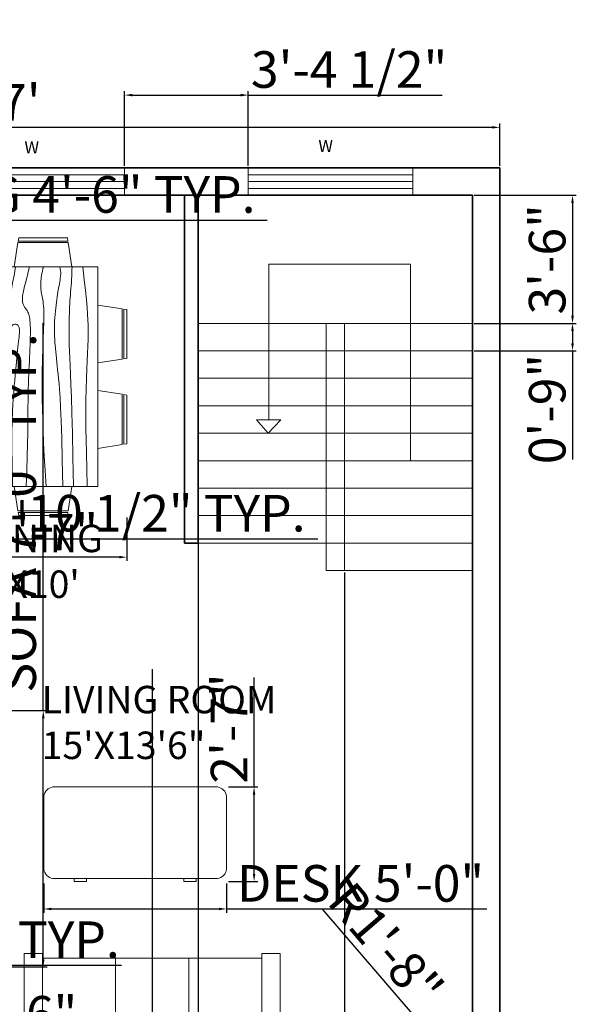
# Model space of a CAD drawing. Units: inches. Extents: x 2691 to 3133, y 1294 to 1993.
# Tile 7 of 7: x 2935 to 3117, y 1606 to 1929. Entities that reach past the tile are written whole.
import ezdxf

# ---------------------------------------------------------------- set-up
doc = ezdxf.new("R2010")
doc.units = ezdxf.units.IN
for name, color, linetype, lineweight in [('A-ANNO-DIMS', 2, 'Continuous', 18), ('A-ANNO-SYMB', 7, 'Continuous', 18), ('A-ANNO-TEXT', 7, 'Continuous', 18), ('A-AREA-IDEN', 7, 'Continuous', 25), ('A-FLOR-STRS', 7, 'Continuous', 18), ('A-FURN', 8, 'Continuous', 18), ('A-GLAZ', 4, 'Continuous', 18), ('A-WALL', 7, 'Continuous', 35)]:
    doc.layers.add(name, color=color, linetype=linetype, lineweight=lineweight)
doc.styles.get("Standard").update_dxf_attribs({"font": 'arial.ttf'})
doc.dimstyles.new('ISO-25', dxfattribs={"dimtxt": 12, "dimasz": 2.5, "dimexe": 1.25, "dimexo": 0.625, "dimtad": 1, "dimdec": 1, "dimlunit": 3, "dimtxsty": 'Standard', "dimcen": 2.5, "dimadec": 0, "dimazin": 0, "dimtfac": 1, "dimtdec": 1, "dimtmove": 0, "dimatfit": 3, "dimfxl": 1, "dimarcsym": 0})

# ---------------------------------------------------------------- blocks, each defined once
blk = doc.blocks.new('Window - Wood Frame 36 in. Wide plan')
for p, q in [((0, 6), (0, 0)), ((0, 4.5), (36, 4.5)), ((36, 6), (36, 0)), ((0, 3), (36, 3)), ((0, 1.5), (36, 1.5))]:
    blk.add_line(p, q)
blk = doc.blocks.new('Sofa - Roundback 7 ft.')
for p, q in [((-12.00002, -32.4421), (-12.00003, -6.5971)), ((11.99997, -32.4421), (11.99998, -6.5971)), ((-36.000027, -34), (-36.000027, -11.4696)), ((35.99998, -34), (35.99998, -11.4696)), ((-35.999844, -13.3819), (35.9998, -13.3819)), ((-36.000027, -32.4421), (35.99998, -32.4421))]:
    blk.add_line(p, q)
for points in [[(-36.000027, -34), (-42.000027, -34), (-42.000027, -8)], [(41.99998, -8), (41.99998, -34), (35.99998, -34)]]:
    blk.add_lwpolyline(points)
for centre, radius, start, end in [((0, -114.25), 114.25, 68.43141, 111.5686), ((-0.00001, -127.1968), 121.1968, 72.72033, 107.2797)]:
    blk.add_arc(centre, radius, start, end)
blk = doc.blocks.new('Desk - 30 x 60 in.')
for p, q in [((-26.999995, 0), (26.999995, 0)), ((-29.999995, -27), (-29.999995, -3)), ((29.999995, -3), (29.999995, -27)), ((26.999995, -30), (-26.999995, -30)), ((-20.000005, -30), (-20.000005, -31)), ((-20.000005, -31), (-16.000005, -31)), ((-16.000005, -31), (-16.000005, -30)), ((15.999995, -31), (15.999995, -30)), ((19.999995, -31), (15.999995, -31)), ((19.999995, -30), (19.999995, -31))]:
    blk.add_line(p, q)
for centre, start, end in [((-26.499995, -3.5), 98.1301, 171.8699), ((26.499995, -3.5), 8.130102, 81.8699), ((-26.499995, -26.5), 188.1301, 261.8699), ((26.499995, -26.5), 278.1301, 351.8699)]:
    blk.add_arc(centre, 3.535534, start, end)
blk = doc.blocks.new('Dining Set - 36 x 72 in.')
for p, q in [((-22.2343, 26.00059), (-23.4847, 17.99762)), ((-22.2304, 26), (-5.7608, 26)), ((-22, 27.5), (-22.1562, 26.50042)), ((-5.8416, 26.5), (-22.1534, 26.5)), ((-22, 27.5), (-6, 27.5)), ((-5.8437, 26.49966), (-6, 27.5)), ((-4.5152, 17.99762), (-5.7655, 25.99926)), ((5.7657, 26.00059), (4.5153, 17.99762)), ((5.7696, 26), (22.2392, 26)), ((6, 27.5), (5.8438, 26.50042)), ((22.1584, 26.5), (5.8466, 26.5)), ((6, 27.5), (22, 27.5)), ((22.1563, 26.49966), (22, 27.5)), ((23.4848, 17.99762), (22.2345, 25.99926)), ((36, 18), (-36, 18)), ((-36, 18), (-36, -18)), ((36, -18), (36, 18)), ((-45.5, 8), (-44.5004, 8.15617)), ((-45.5, 8), (-45.5, -8)), ((-44.5, -8.15843), (-44.5, 8.15338)), ((-44.0006, 8.23428), (-35.9976, 9.48474)), ((-44, 8.23041), (-44, -8.23915)), ((44.0006, 8.23428), (35.9976, 9.48474)), ((44, 8.23041), (44, -8.23915)), ((44.5, -8.15843), (44.5, 8.15338)), ((45.5, 8), (44.5005, 8.15617)), ((45.5, 8), (45.5, -8)), ((-44.4997, -8.15631), (-45.5, -8)), ((-35.9976, -9.48476), (-43.9993, -8.2345)), ((35.9976, -9.48476), (43.9993, -8.2345)), ((44.4997, -8.15631), (45.5, -8)), ((-36, -18), (36, -18)), ((-22.2343, -26.0006), (-23.4847, -17.99762)), ((-4.5152, -17.99762), (-5.7655, -25.99928)), ((5.7657, -26.0006), (4.5153, -17.99762)), ((23.4848, -17.99762), (22.2345, -25.99928)), ((-22.2304, -26), (-5.7608, -26)), ((-22, -27.5), (-22.1562, -26.50044)), ((-5.8416, -26.5), (-22.1534, -26.5)), ((-22, -27.5), (-6, -27.5)), ((-5.8437, -26.49967), (-6, -27.5)), ((5.7696, -26), (22.2392, -26)), ((6, -27.5), (5.8438, -26.50044)), ((22.1584, -26.5), (5.8466, -26.5)), ((6, -27.5), (22, -27.5)), ((22.1563, -26.49967), (22, -27.5))]:
    blk.add_line(p, q)
for points in [[(-36, 15), (-31.1772, 14.97754), (-26.8079, 14.91406), (-22.8538, 14.81543), (-19.276, 14.6875), (-16.0362, 14.53613), (-13.0957, 14.36718), (-10.4159, 14.18652), (-7.9583, 14), (-5.6904, 13.81315), (-3.6035, 13.63021), (-1.6954, 13.45508), (0.0365, 13.29166), (1.5945, 13.14388), (2.9811, 13.01562), (4.1988, 12.9108), (5.25, 12.83333), (6.1393, 12.78613), (6.8802, 12.76823), (7.4883, 12.77767), (7.9792, 12.8125), (8.3685, 12.87077), (8.6719, 12.95052), (8.9049, 13.0498), (9.0833, 13.16666), (9.2205, 13.29899), (9.3216, 13.44401), (9.3895, 13.59879), (9.4271, 13.76041), (9.4373, 13.92594), (9.4232, 14.09245), (9.3875, 14.257), (9.3333, 14.41666), (9.2638, 14.56917), (9.1836, 14.71484), (9.0975, 14.85465), (9.0104, 14.98958), (8.9272, 15.1206), (8.8529, 15.2487), (8.7922, 15.37483), (8.75, 15.5), (8.7305, 15.62467), (8.7344, 15.74739), (8.7617, 15.86621), (8.8125, 15.97916), (8.8867, 16.08431), (8.9844, 16.17968), (9.1055, 16.26334), (9.25, 16.33333), (9.4189, 16.38802), (9.6172, 16.42708), (9.8506, 16.45052), (10.125, 16.45833), (10.4463, 16.45052), (10.8203, 16.42708), (11.2529, 16.38802), (11.75, 16.33333), (12.3184, 16.26318), (12.9694, 16.17838), (13.7151, 16.07991), (14.5677, 15.96875), (15.5395, 15.84586), (16.6426, 15.71224), (17.8893, 15.56884), (19.2917, 15.41666), (20.859, 15.25667), (22.5879, 15.08984), (24.4721, 14.91715), (26.5052, 14.73958), (28.6809, 14.5581), (30.9929, 14.3737), (33.4347, 14.18733), (36, 14)], [(-36, 10), (-28.9766, 10.14274), (-23.1725, 10.20442), (-18.4241, 10.19775), (-14.5677, 10.13541), (-11.4399, 10.03011), (-8.877, 9.89453), (-6.7154, 9.74137), (-4.7917, 9.58333), (-2.9698, 9.43082), (-1.2246, 9.28515), (0.4415, 9.14534), (2.026, 9.01041), (3.5266, 8.87939), (4.9408, 8.7513), (6.266, 8.62516), (7.5, 8.5), (8.6411, 8.37549), (9.6914, 8.2539), (10.6538, 8.13818), (11.5312, 8.03125), (12.3267, 7.93603), (13.043, 7.85547), (13.6831, 7.79248), (14.25, 7.75), (14.7471, 7.7303), (15.1797, 7.73307), (15.5537, 7.75732), (15.875, 7.80208), (16.1494, 7.86637), (16.3828, 7.94922), (16.5811, 8.04964), (16.75, 8.16666), (16.8944, 8.29915), (17.0143, 8.44531), (17.1089, 8.60319), (17.1771, 8.77083), (17.218, 8.94629), (17.2305, 9.1276), (17.2137, 9.31282), (17.1667, 9.5), (17.0895, 9.6875), (16.987, 9.875), (16.8649, 10.0625), (16.7292, 10.25), (16.5856, 10.4375), (16.4401, 10.625), (16.2985, 10.8125), (16.1667, 11), (16.05, 11.18733), (15.9518, 11.3737), (15.8752, 11.5581), (15.8229, 11.73958), (15.798, 11.91715), (15.8034, 12.08984), (15.842, 12.25667), (15.9167, 12.41666), (16.0295, 12.56836), (16.1784, 12.70833), (16.3605, 12.83268), (16.5729, 12.9375), (16.8127, 13.01888), (17.0768, 13.07291), (17.3625, 13.0957), (17.6667, 13.08333), (17.9894, 13.03312), (18.3418, 12.94726), (18.7382, 12.82918), (19.1927, 12.68229), (19.7195, 12.51001), (20.3327, 12.31575), (21.0465, 12.10294), (21.875, 11.875), (22.8357, 11.63354), (23.959, 11.37304), (25.2786, 11.08618), (26.8282, 10.76562), (28.6414, 10.40405), (30.752, 9.99414), (33.1936, 9.52856), (36, 9)], [(-36, 5.5), (-30.7157, 5.3348), (-26.069, 5.20963), (-21.9946, 5.11767), (-18.4271, 5.05208), (-15.3009, 5.00602), (-12.5508, 4.97265), (-10.1112, 4.94515), (-7.9167, 4.91666), (-5.909, 4.88167), (-4.0586, 4.83984), (-2.3429, 4.79215), (-0.7396, 4.73958), (0.7739, 4.6831), (2.22, 4.6237), (3.6213, 4.56233), (5, 4.5), (6.373, 4.43782), (7.7344, 4.3776), (9.0723, 4.32129), (10.375, 4.27083), (11.6309, 4.22819), (12.8281, 4.19531), (13.9551, 4.17415), (15, 4.16666), (15.954, 4.17448), (16.819, 4.19791), (17.6001, 4.23698), (18.3021, 4.29166), (18.9299, 4.36198), (19.4883, 4.44791), (19.9823, 4.54948), (20.4167, 4.66666), (20.7969, 4.79899), (21.1302, 4.94401), (21.4245, 5.09879), (21.6875, 5.26041), (21.9271, 5.42594), (22.1511, 5.59245), (22.3672, 5.757), (22.5834, 5.91666), (22.8065, 6.06868), (23.0404, 6.21093), (23.2879, 6.34147), (23.5521, 6.45833), (23.8358, 6.55957), (24.142, 6.64323), (24.4735, 6.70735), (24.8334, 6.75), (25.2235, 6.76969), (25.642, 6.76692), (26.0858, 6.74267), (26.5521, 6.69791), (27.0379, 6.63362), (27.5404, 6.55078), (28.0565, 6.45036), (28.5834, 6.33333), (29.1242, 6.19987), (29.7071, 6.04687), (30.3661, 5.87044), (31.1354, 5.66666), (32.0493, 5.43164), (33.142, 5.16146), (34.4475, 4.85221), (36, 4.5)], [(-36, -1), (-30.7915, -0.6591), (-26.0195, -0.38216), (-21.6519, -0.16284), (-17.6563, 0.00521), (-14.0005, 0.12833), (-10.6523, 0.21289), (-7.5796, 0.26522), (-4.75, 0.29166), (-2.134, 0.29793), (0.2878, 0.28711), (2.5317, 0.26163), (4.6146, 0.22396), (6.5529, 0.17651), (8.3633, 0.12174), (10.0623, 0.06209), (11.6667, 0), (13.1899, -0.06201), (14.6341, -0.1211), (15.9982, -0.17432), (17.2813, -0.21875), (18.4823, -0.25147), (19.6003, -0.26953), (20.6343, -0.27002), (21.5834, -0.25), (22.4481, -0.20768), (23.2357, -0.14584), (23.9549, -0.06836), (24.6146, 0.02083), (25.2235, 0.11784), (25.7904, 0.21875), (26.3241, 0.31966), (26.8334, 0.41666), (27.3265, 0.50618), (27.8099, 0.58593), (28.2894, 0.65397), (28.7709, 0.70833), (29.2601, 0.74707), (29.763, 0.76823), (30.2855, 0.76985), (30.8334, 0.75), (31.4088, 0.70784), (31.9994, 0.64713), (32.589, 0.57275), (33.1615, 0.48958), (33.7008, 0.4025), (34.1908, 0.3164), (34.6153, 0.23616), (34.9584, 0.16666), (35.2099, 0.11165), (35.3848, 0.07031), (35.504, 0.04069), (35.5886, 0.02083), (35.6594, 0.00879), (35.7377, 0.0026), (35.8442, 0.00032), (36, 0)], [(-36, -6.5), (-27.1843, -6.31267), (-20.084, -6.1263), (-14.469, -5.9419), (-10.1094, -5.76042), (-6.7752, -5.58285), (-4.2363, -5.41016), (-2.2629, -5.24333), (-0.625, -5.08334), (0.8708, -4.93099), (2.2715, -4.78646), (3.5872, -4.64974), (4.8281, -4.52084), (6.0046, -4.39974), (7.127, -4.28646), (8.2053, -4.18099), (9.25, -4.08334), (10.2705, -3.99382), (11.2734, -3.91407), (12.2647, -3.84603), (13.25, -3.79167), (14.2354, -3.75293), (15.2266, -3.73177), (16.2295, -3.73015), (17.25, -3.75), (18.2912, -3.79248), (19.3451, -3.85547), (20.4009, -3.93604), (21.4479, -4.03125), (22.4754, -4.13819), (23.4727, -4.25391), (24.4289, -4.37549), (25.3334, -4.5), (26.1785, -4.62492), (26.9694, -4.74935), (27.7145, -4.87281), (28.4219, -4.99479), (29.1, -5.11483), (29.7572, -5.23242), (30.4016, -5.34709), (31.0417, -5.45834), (31.6837, -5.56437), (32.3262, -5.65821), (32.9658, -5.73153), (33.599, -5.77604), (34.2224, -5.78345), (34.8327, -5.74545), (35.4264, -5.65373), (36, -5.5)], [(-36, -10), (-26.4022, -9.81299), (-18.4675, -9.62891), (-11.9839, -9.45069), (-6.7396, -9.28125), (-2.5226, -9.12354), (0.8789, -8.98047), (3.6769, -8.85498), (6.0833, -8.75), (8.2767, -8.66765), (10.3021, -8.60677), (12.1712, -8.56543), (13.8958, -8.54167), (15.4876, -8.53353), (16.9583, -8.53907), (18.3197, -8.55632), (19.5834, -8.58334), (20.7616, -8.61841), (21.8685, -8.66081), (22.9188, -8.71004), (23.9271, -8.76563), (24.9081, -8.82707), (25.8763, -8.89388), (26.8465, -8.96558), (27.8334, -9.04167), (28.8474, -9.12118), (29.8828, -9.20117), (30.93, -9.27824), (31.9792, -9.34896), (33.0205, -9.40991), (34.0443, -9.45768), (35.0407, -9.48885), (36, -9.5)], [(-36, -14.5), (-30.0881, -14.33513), (-25.0332, -14.21224), (-20.7312, -14.12647), (-17.0781, -14.07292), (-13.97, -14.04671), (-11.3027, -14.04297), (-8.9724, -14.05681), (-6.875, -14.08334), (-4.9224, -14.11833), (-3.0905, -14.16016), (-1.3709, -14.20785), (0.2448, -14.26042), (1.7647, -14.3169), (3.1973, -14.3763), (4.5507, -14.43767), (5.8333, -14.5), (7.0554, -14.5621), (8.235, -14.62175), (9.3922, -14.67652), (10.5469, -14.72396), (11.7192, -14.76164), (12.929, -14.78711), (14.1965, -14.79794), (15.5417, -14.79167), (16.9933, -14.76424), (18.6152, -14.70508), (20.4804, -14.60197), (22.6615, -14.44271), (25.2312, -14.21509), (28.2624, -13.9069), (31.8277, -13.50594), (36, -13)]]:
    blk.add_lwpolyline(points)
blk = doc.blocks.new('*D10')
at = {"layer": 'A-ANNO-DIMS', "color": 0, "lineweight": -2, "transparency": 16777216}
for p, q in [((2768.25, 1880.68), (2768.25, 1894.58)), ((3089.75, 1893.33), (2770.75, 1893.33)), ((3092.25, 1880.68), (3092.25, 1894.58))]:
    blk.add_line(p, q, dxfattribs=at)
at = {"layer": 'A-ANNO-DIMS', "color": 0, "transparency": 16777216}
for points in [[(2770.75, 1893.75), (2770.75, 1892.92), (2768.25, 1893.33)], [(3089.75, 1893.75), (3089.75, 1892.92), (3092.25, 1893.33)]]:
    blk.add_solid(points, dxfattribs=at)
at = {"layer": 'Defpoints', "color": 0, "transparency": 16777216}
for p in [(2768.25, 1893.33), (2768.25, 1880.05), (3092.25, 1880.05)]:
    blk.add_point(p, dxfattribs=at)
at = {"layer": 'A-ANNO-DIMS', "color": 0, "transparency": 16777216, "insert": (2930.25, 1899.98), "char_height": 12, "attachment_point": 5}
blk.add_mtext("27'", dxfattribs=at)
blk = doc.blocks.new('*D14')
at = {"layer": 'A-ANNO-DIMS', "color": 0, "lineweight": -2, "transparency": 16777216}
for p, q in [((2806.97, 1870.43), (2806.97, 1861.7)), ((2860.97, 1870.43), (2860.97, 1861.7)), ((2809.47, 1862.95), (2858.47, 1862.95)), ((2860.97, 1862.95), (3015.92, 1862.95))]:
    blk.add_line(p, q, dxfattribs=at)
at = {"layer": 'A-ANNO-DIMS', "color": 0, "transparency": 16777216}
for points in [[(2809.47, 1863.37), (2809.47, 1862.54), (2806.97, 1862.95)], [(2858.47, 1863.37), (2858.47, 1862.54), (2860.97, 1862.95)]]:
    blk.add_solid(points, dxfattribs=at)
at = {"layer": 'Defpoints', "color": 0, "transparency": 16777216}
for p in [(2806.97, 1871.05), (2860.97, 1871.05), (2860.97, 1862.95)]:
    blk.add_point(p, dxfattribs=at)
at = {"layer": 'A-ANNO-DIMS', "color": 0, "transparency": 16777216, "insert": (2939.69, 1869.78), "char_height": 12, "attachment_point": 5}
blk.add_mtext('GLAZING 4\'-6" TYP.', dxfattribs=at)
blk = doc.blocks.new('*D16')
at = {"layer": 'A-ANNO-DIMS', "color": 0, "lineweight": -2, "transparency": 16777216}
for p, q in [((2957.85, 1586.68), (2957.85, 1595.4)), ((3011.85, 1586.68), (3011.85, 1595.4)), ((2957.85, 1594.15), (2844.15, 1594.15)), ((3009.35, 1594.15), (2960.35, 1594.15))]:
    blk.add_line(p, q, dxfattribs=at)
at = {"layer": 'A-ANNO-DIMS', "color": 0, "transparency": 16777216}
for points in [[(2960.35, 1594.57), (2960.35, 1593.74), (2957.85, 1594.15)], [(3009.35, 1594.57), (3009.35, 1593.74), (3011.85, 1594.15)]]:
    blk.add_solid(points, dxfattribs=at)
at = {"layer": 'Defpoints', "color": 0, "transparency": 16777216}
for p in [(2957.85, 1594.15), (2957.85, 1586.05), (3011.85, 1586.05)]:
    blk.add_point(p, dxfattribs=at)
at = {"layer": 'A-ANNO-DIMS', "color": 0, "transparency": 16777216, "insert": (2899.75, 1600.98), "char_height": 12, "attachment_point": 5}
blk.add_mtext('GLAZING 4\'-6"', dxfattribs=at)
blk = doc.blocks.new('*D20')
at = {"layer": 'A-ANNO-DIMS', "color": 0, "lineweight": -2, "transparency": 16777216}
for p, q in [((2942.46, 1702.1), (2942.46, 1829.23)), ((2930.49, 1702.1), (2943.71, 1702.1)), ((2942.46, 1620.6), (2942.46, 1699.6)), ((2930.49, 1618.1), (2943.71, 1618.1))]:
    blk.add_line(p, q, dxfattribs=at)
at = {"layer": 'A-ANNO-DIMS', "color": 0, "transparency": 16777216}
for points in [[(2942.05, 1699.6), (2942.88, 1699.6), (2942.46, 1702.1)], [(2942.05, 1620.6), (2942.88, 1620.6), (2942.46, 1618.1)]]:
    blk.add_solid(points, dxfattribs=at)
at = {"layer": 'Defpoints', "color": 0, "transparency": 16777216}
for p in [(2929.86, 1702.1), (2942.46, 1702.1), (2929.86, 1618.1)]:
    blk.add_point(p, dxfattribs=at)
at = {"layer": 'A-ANNO-DIMS', "color": 0, "transparency": 16777216, "insert": (2935.63, 1766.91), "char_height": 12, "attachment_point": 5, "rotation": 90}
blk.add_mtext('SOFA 7\'-0" TYP.', dxfattribs=at)
blk = doc.blocks.new('*D24')
at = {"layer": 'A-ANNO-DIMS', "color": 0, "lineweight": -2, "transparency": 16777216}
for p, q in [((2823.75, 1755.69), (2823.75, 1759.69)), ((2846.25, 1755.69), (2846.25, 1759.69)), ((2826.25, 1758.44), (2843.75, 1758.44)), ((2846.25, 1758.44), (3032.5, 1758.44))]:
    blk.add_line(p, q, dxfattribs=at)
at = {"layer": 'A-ANNO-DIMS', "color": 0, "transparency": 16777216}
for points in [[(2826.25, 1758.86), (2826.25, 1758.02), (2823.75, 1758.44)], [(2843.75, 1758.86), (2843.75, 1758.02), (2846.25, 1758.44)]]:
    blk.add_solid(points, dxfattribs=at)
at = {"layer": 'Defpoints', "color": 0, "transparency": 16777216}
for p in [(2846.25, 1758.44), (2823.75, 1755.06), (2846.25, 1755.06)]:
    blk.add_point(p, dxfattribs=at)
at = {"layer": 'A-ANNO-DIMS', "color": 0, "transparency": 16777216, "insert": (2940.63, 1765.27), "char_height": 12, "attachment_point": 5}
blk.add_mtext('D1 LEAF 1\'-10 1/2" TYP.', dxfattribs=at)
blk = doc.blocks.new('*D27')
at = {"layer": 'A-ANNO-DIMS', "color": 0, "lineweight": -2, "transparency": 16777216}
for p, q in [((2886.75, 1621.43), (2886.75, 1617.43)), ((2888.75, 1621.43), (2888.75, 1617.43)), ((2884.25, 1618.68), (2881.75, 1618.68)), ((2886.75, 1618.68), (2888.75, 1618.68)), ((2891.25, 1618.68), (2968.15, 1618.68))]:
    blk.add_line(p, q, dxfattribs=at)
at = {"layer": 'A-ANNO-DIMS', "color": 0, "transparency": 16777216}
for points in [[(2884.25, 1619.1), (2884.25, 1618.26), (2886.75, 1618.68)], [(2891.25, 1619.1), (2891.25, 1618.26), (2888.75, 1618.68)]]:
    blk.add_solid(points, dxfattribs=at)
at = {"layer": 'Defpoints', "color": 0, "transparency": 16777216}
for p in [(2886.75, 1622.05), (2888.75, 1622.05), (2888.75, 1618.68)]:
    blk.add_point(p, dxfattribs=at)
at = {"layer": 'A-ANNO-DIMS', "color": 0, "transparency": 16777216, "insert": (2930.95, 1625.43), "char_height": 12, "attachment_point": 5}
blk.add_mtext('0\'-2" TYP.', dxfattribs=at)
blk = doc.blocks.new('*D28')
at = {"layer": 'A-ANNO-DIMS', "color": 0, "lineweight": -2, "transparency": 16777216}
for p, q in [((2942.63, 1645.44), (2942.63, 1635.82)), ((3002.63, 1645.44), (3002.63, 1635.82)), ((2945.13, 1637.07), (3000.13, 1637.07)), ((3002.63, 1637.07), (3087.99, 1637.07))]:
    blk.add_line(p, q, dxfattribs=at)
at = {"layer": 'A-ANNO-DIMS', "color": 0, "transparency": 16777216}
for points in [[(2945.13, 1637.48), (2945.13, 1636.65), (2942.63, 1637.07)], [(3000.13, 1637.48), (3000.13, 1636.65), (3002.63, 1637.07)]]:
    blk.add_solid(points, dxfattribs=at)
at = {"layer": 'Defpoints', "color": 0, "transparency": 16777216}
for p in [(2942.63, 1646.07), (3002.63, 1646.07), (3002.63, 1637.07)]:
    blk.add_point(p, dxfattribs=at)
at = {"layer": 'A-ANNO-DIMS', "color": 0, "transparency": 16777216, "insert": (3046.56, 1643.9), "char_height": 12, "attachment_point": 5}
blk.add_mtext('DESK 5\'-0"', dxfattribs=at)
blk = doc.blocks.new('*D29')
at = {"layer": 'A-ANNO-DIMS', "color": 0, "lineweight": -2, "transparency": 16777216}
for p, q in [((3011.63, 1677.07), (3011.63, 1712.92)), ((3003.25, 1677.07), (3012.88, 1677.07)), ((3011.63, 1648.57), (3011.63, 1674.57)), ((3003.25, 1646.07), (3012.88, 1646.07))]:
    blk.add_line(p, q, dxfattribs=at)
at = {"layer": 'A-ANNO-DIMS', "color": 0, "transparency": 16777216}
for points in [[(3011.21, 1674.57), (3012.04, 1674.57), (3011.63, 1677.07)], [(3011.21, 1648.57), (3012.04, 1648.57), (3011.63, 1646.07)]]:
    blk.add_solid(points, dxfattribs=at)
at = {"layer": 'Defpoints', "color": 0, "transparency": 16777216}
for p in [(3002.63, 1677.07), (3011.63, 1677.07), (3002.63, 1646.07)]:
    blk.add_point(p, dxfattribs=at)
at = {"layer": 'A-ANNO-DIMS', "color": 0, "transparency": 16777216, "insert": (3004.98, 1696.24), "char_height": 12, "attachment_point": 5, "rotation": 90}
blk.add_mtext('2\'-7"', dxfattribs=at)
blk = doc.blocks.new('*D31')
at = {"layer": 'A-ANNO-DIMS', "color": 0, "lineweight": -2, "transparency": 16777216}
for p, q in [((2914.9, 1765.45), (2914.9, 1751.17)), ((2969.9, 1765.45), (2969.9, 1751.17)), ((2967.4, 1752.42), (2917.4, 1752.42))]:
    blk.add_line(p, q, dxfattribs=at)
at = {"layer": 'A-ANNO-DIMS', "color": 0, "transparency": 16777216}
for points in [[(2917.4, 1752.84), (2917.4, 1752), (2914.9, 1752.42)], [(2967.4, 1752.84), (2967.4, 1752), (2969.9, 1752.42)]]:
    blk.add_solid(points, dxfattribs=at)
at = {"layer": 'Defpoints', "color": 0, "transparency": 16777216}
for p in [(2914.9, 1766.07), (2969.9, 1766.07), (2914.9, 1752.42)]:
    blk.add_point(p, dxfattribs=at)
at = {"layer": 'A-ANNO-DIMS', "color": 0, "transparency": 16777216, "insert": (2942.4, 1759.05), "char_height": 12, "attachment_point": 5}
blk.add_mtext('4\'-7"', dxfattribs=at)
blk = doc.blocks.new('*D40')
at = {"layer": 'A-ANNO-DIMS', "color": 0, "lineweight": -2, "transparency": 16777216}
for p, q in [((2969.15, 1880.68), (2969.15, 1905.15)), ((3009.74, 1880.68), (3009.74, 1905.15)), ((2971.65, 1903.9), (3007.24, 1903.9)), ((3009.74, 1903.9), (3073.35, 1903.9))]:
    blk.add_line(p, q, dxfattribs=at)
at = {"layer": 'A-ANNO-DIMS', "color": 0, "transparency": 16777216}
for points in [[(2971.65, 1904.32), (2971.65, 1903.49), (2969.15, 1903.9)], [(3007.24, 1904.32), (3007.24, 1903.49), (3009.74, 1903.9)]]:
    blk.add_solid(points, dxfattribs=at)
at = {"layer": 'Defpoints', "color": 0, "transparency": 16777216}
for p in [(3009.74, 1903.9), (2969.15, 1880.05), (3009.74, 1880.05)]:
    blk.add_point(p, dxfattribs=at)
at = {"layer": 'A-ANNO-DIMS', "color": 0, "transparency": 16777216, "insert": (3042.8, 1910.74), "char_height": 12, "attachment_point": 5}
blk.add_mtext('3\'-4 1/2"', dxfattribs=at)
blk = doc.blocks.new('*D49')
at = {"layer": 'A-ANNO-DIMS', "color": 0, "lineweight": -2, "transparency": 16777216}
for p, q in [((2993.25, 1870.43), (2993.25, 1398.95)), ((3083.25, 1870.43), (3083.25, 1398.95)), ((2995.75, 1400.2), (3080.75, 1400.2))]:
    blk.add_line(p, q, dxfattribs=at)
at = {"layer": 'A-ANNO-DIMS', "color": 0, "transparency": 16777216}
for points in [[(2995.75, 1400.62), (2995.75, 1399.79), (2993.25, 1400.2)], [(3080.75, 1400.62), (3080.75, 1399.79), (3083.25, 1400.2)]]:
    blk.add_solid(points, dxfattribs=at)
at = {"layer": 'Defpoints', "color": 0, "transparency": 16777216}
for p in [(2993.25, 1871.05), (3083.25, 1871.05), (3083.25, 1400.2)]:
    blk.add_point(p, dxfattribs=at)
at = {"layer": 'A-ANNO-DIMS', "color": 0, "transparency": 16777216, "insert": (3038.25, 1406.96), "char_height": 12, "attachment_point": 5}
blk.add_mtext('7\'-6"', dxfattribs=at)
blk = doc.blocks.new('*D50')
at = {"layer": 'A-ANNO-DIMS', "color": 0, "lineweight": -2, "transparency": 16777216}
for p, q in [((3083.87, 1871.05), (3117.35, 1871.05)), ((3116.1, 1868.55), (3116.1, 1831.55)), ((3083.87, 1829.05), (3117.35, 1829.05))]:
    blk.add_line(p, q, dxfattribs=at)
at = {"layer": 'A-ANNO-DIMS', "color": 0, "transparency": 16777216}
for points in [[(3115.68, 1868.55), (3116.52, 1868.55), (3116.1, 1871.05)], [(3115.68, 1831.55), (3116.52, 1831.55), (3116.1, 1829.05)]]:
    blk.add_solid(points, dxfattribs=at)
at = {"layer": 'Defpoints', "color": 0, "transparency": 16777216}
for p in [(3083.25, 1871.05), (3083.25, 1829.05), (3116.1, 1829.05)]:
    blk.add_point(p, dxfattribs=at)
at = {"layer": 'A-ANNO-DIMS', "color": 0, "transparency": 16777216, "insert": (3109.34, 1850.05), "char_height": 12, "attachment_point": 5, "rotation": 90}
blk.add_mtext('3\'-6"', dxfattribs=at)
blk = doc.blocks.new('*D51')
at = {"layer": 'A-ANNO-DIMS', "color": 0, "lineweight": -2, "transparency": 16777216}
for p, q in [((3083.87, 1829.05), (3117.35, 1829.05)), ((3116.1, 1826.55), (3116.1, 1822.55)), ((3083.87, 1820.05), (3117.35, 1820.05)), ((3116.1, 1820.05), (3116.1, 1784.41))]:
    blk.add_line(p, q, dxfattribs=at)
at = {"layer": 'A-ANNO-DIMS', "color": 0, "transparency": 16777216}
for points in [[(3115.68, 1826.55), (3116.52, 1826.55), (3116.1, 1829.05)], [(3115.68, 1822.55), (3116.52, 1822.55), (3116.1, 1820.05)]]:
    blk.add_solid(points, dxfattribs=at)
at = {"layer": 'Defpoints', "color": 0, "transparency": 16777216}
for p in [(3083.25, 1829.05), (3083.25, 1820.05), (3116.1, 1820.05)]:
    blk.add_point(p, dxfattribs=at)
at = {"layer": 'A-ANNO-DIMS', "color": 0, "transparency": 16777216, "insert": (3109.35, 1800.98), "char_height": 12, "attachment_point": 5, "rotation": 90}
blk.add_mtext('0\'-9"', dxfattribs=at)
blk = doc.blocks.new('*D52')
at = {"layer": 'A-ANNO-DIMS', "color": 0, "lineweight": -2, "transparency": 16777216}
for p, q in [((3041.25, 1747.43), (3041.25, 1398.95)), ((3083.25, 1747.43), (3083.25, 1398.95)), ((3043.75, 1400.2), (3080.75, 1400.2))]:
    blk.add_line(p, q, dxfattribs=at)
at = {"layer": 'A-ANNO-DIMS', "color": 0, "transparency": 16777216}
for points in [[(3043.75, 1400.62), (3043.75, 1399.79), (3041.25, 1400.2)], [(3080.75, 1400.62), (3080.75, 1399.79), (3083.25, 1400.2)]]:
    blk.add_solid(points, dxfattribs=at)
at = {"layer": 'Defpoints', "color": 0, "transparency": 16777216}
for p in [(3041.25, 1748.05), (3083.25, 1748.05), (3083.25, 1400.2)]:
    blk.add_point(p, dxfattribs=at)
at = {"layer": 'A-ANNO-DIMS', "color": 0, "transparency": 16777216, "insert": (3062.25, 1406.96), "char_height": 12, "attachment_point": 5}
blk.add_mtext('3\'-6"', dxfattribs=at)
blk = doc.blocks.new('*D62')
at = {"layer": 'A-ANNO-DIMS', "color": 0, "lineweight": -2, "transparency": 16777216}
for p, q in [((3034.07, 1636.88), (3064.78, 1601.13)), ((3079.48, 1584.03), (3066.41, 1599.24))]:
    blk.add_line(p, q, dxfattribs=at)
at = {"layer": 'A-ANNO-DIMS', "color": 0, "transparency": 16777216}
blk.add_solid([(3065.1, 1601.4), (3064.47, 1600.86), (3066.41, 1599.24)], dxfattribs=at)
at = {"layer": 'Defpoints', "color": 0, "transparency": 16777216}
for p in [(3066.41, 1599.24), (3079.48, 1584.03)]:
    blk.add_point(p, dxfattribs=at)
at = {"layer": 'A-ANNO-DIMS', "color": 0, "transparency": 16777216, "insert": (3053.73, 1624.36), "char_height": 12, "attachment_point": 5, "rotation": 310.6735}
blk.add_mtext('R1\'-8"', dxfattribs=at)
blk = doc.blocks.new('*D66')
at = {"layer": 'A-ANNO-DIMS', "color": 0, "lineweight": -2, "transparency": 16777216}
for p, q in [((2978.21, 1715.72), (2978.21, 1594.52)), ((2978.21, 1481.83), (2978.21, 1592.02))]:
    blk.add_line(p, q, dxfattribs=at)
at = {"layer": 'A-ANNO-DIMS', "color": 0, "transparency": 16777216}
blk.add_solid([(2977.79, 1592.02), (2978.62, 1592.02), (2978.21, 1594.52)], dxfattribs=at)
at = {"layer": 'Defpoints', "color": 0, "transparency": 16777216}
for p in [(2978.21, 1715.72), (2978.21, 1594.52)]:
    blk.add_point(p, dxfattribs=at)
at = {"layer": 'A-ANNO-DIMS', "color": 0, "transparency": 16777216, "insert": (2971.46, 1521.8), "char_height": 12, "attachment_point": 5, "rotation": 89.9999}
blk.add_mtext('2X R10\'-1"', dxfattribs=at)
blk = doc.blocks.new('*D67')
at = {"layer": 'A-ANNO-DIMS', "color": 0, "lineweight": -2, "transparency": 16777216}
for p, q in [((2978.21, 1702.77), (2978.21, 1588.52)), ((2978.21, 1470.68), (2978.21, 1586.02))]:
    blk.add_line(p, q, dxfattribs=at)
at = {"layer": 'A-ANNO-DIMS', "color": 0, "transparency": 16777216}
blk.add_solid([(2977.79, 1586.02), (2978.62, 1586.02), (2978.21, 1588.52)], dxfattribs=at)
at = {"layer": 'Defpoints', "color": 0, "transparency": 16777216}
for p in [(2978.21, 1702.77), (2978.21, 1588.52)]:
    blk.add_point(p, dxfattribs=at)
at = {"layer": 'A-ANNO-DIMS', "color": 0, "transparency": 16777216, "insert": (2971.38, 1519.97), "char_height": 12, "attachment_point": 5, "rotation": 89.9999}
blk.add_mtext('2X R9\'-6 1/2"', dxfattribs=at)

msp = doc.modelspace()

# ---------------------------------------------------------------- linework, layer by layer
at = {"layer": 'A-ANNO-SYMB'}
for p, q in [((3062.99, 1848.52), (3016.42, 1848.52)), ((3016.42, 1848.52), (3016.42, 1797.47)), ((3062.99, 1784.05), (3062.99, 1848.52)), ((3016.42, 1797.47), (3012.42, 1797.47)), ((3012.42, 1797.47), (3016.42, 1797.47)), ((3016.29, 1793.05), (3012.42, 1797.47)), ((3020.42, 1797.47), (3016.29, 1793.05)), ((3016.42, 1797.47), (3020.42, 1797.47))]:
    msp.add_line(p, q, dxfattribs=at)
at = {"layer": 'A-FLOR-STRS'}
for p, q in [((2993.25, 1829.05), (3083.25, 1829.05)), ((3035.25, 1748.05), (3035.25, 1829.05)), ((3041.25, 1748.05), (3041.25, 1829.05)), ((2993.25, 1820.05), (3083.25, 1820.05)), ((2993.25, 1811.05), (3083.25, 1811.05)), ((2993.25, 1802.05), (3083.25, 1802.05)), ((2993.25, 1793.05), (3083.25, 1793.05)), ((2993.25, 1784.05), (3083.25, 1784.05)), ((2993.25, 1775.05), (3083.25, 1775.05)), ((2993.25, 1766.05), (3083.25, 1766.05)), ((2993.25, 1757.05), (3083.25, 1757.05)), ((3035.25, 1748.05), (3083.25, 1748.05))]:
    msp.add_line(p, q, dxfattribs=at)
at = {"layer": 'A-WALL'}
for p, q in [((3092.25, 1880.05), (2768.25, 1880.05)), ((3092.25, 1424.05), (3092.25, 1880.05)), ((3083.25, 1871.05), (2880.75, 1871.05)), ((2988.75, 1871.05), (2988.75, 1757.05)), ((2993.25, 1871.05), (2993.25, 1757.05)), ((3083.25, 1433.05), (3083.25, 1871.05)), ((2993.25, 1757.05), (2988.75, 1757.05))]:
    msp.add_line(p, q, dxfattribs=at)

# ---------------------------------------------------------------- block references
at = {"layer": 'A-FURN'}
for name, p, rotation in [('Dining Set - 36 x 72 in.', (2942.4, 1811.57), 90), ('Sofa - Roundback 7 ft.', (2978.21, 1588.52), 180)]:
    msp.add_blockref(name, p, dxfattribs=dict(at, rotation=rotation))
msp.add_blockref('Desk - 30 x 60 in.', (2972.63, 1677.07), dxfattribs=at)
at = {"layer": 'A-GLAZ', "xscale": 1.5, "yscale": 1.5}
for p in [(2915.15, 1871.05), (3009.74, 1871.05)]:
    msp.add_blockref('Window - Wood Frame 36 in. Wide plan', p, dxfattribs=at)

# ---------------------------------------------------------------- texts
at = {"layer": 'A-ANNO-TEXT', "char_height": 4, "attachment_point": 1}
for insert in [(2936.29, 1888.77), (3032.72, 1889.22)]:
    msp.add_mtext_dynamic_manual_height_columns('W', width=0.1038, gutter_width=12.5, heights=[0], dxfattribs=dict(at, insert=insert))
at = {"layer": 'A-AREA-IDEN', "char_height": 9, "attachment_point": 1}
for s, insert in [("DINING \\P8'X10'", (2920.14, 1763.05)), ('LIVING ROOM \\P15\'X13\'6"', (2941.94, 1710.22))]:
    msp.add_mtext(s, dxfattribs=dict(at, insert=insert))

# ---------------------------------------------------------------- dimensions: what is measured, and where the dimension line sits
at = {"layer": 'A-ANNO-DIMS'}
for base, p1, p2, override, picture, middle in [((3009.74, 1903.9), (2969.15, 1880.05), (3009.74, 1880.05), {"dimdec": 1, "dimlfac": 1, "dimrnd": 0, "dimzin": 1, "dimdsep": 46, "dimlunit": 4, "dimfrac": 2}, '*D40', (3042.8, 1910.74)), ((2768.25, 1893.33), (3092.25, 1880.05), (2768.25, 1880.05), {"dimclrd": 0, "dimclre": 0, "dimclrt": 0}, '*D10', (2930.25, 1899.98)), ((3083.25, 1400.2), (2993.25, 1871.05), (3083.25, 1871.05), {"dimdec": 1, "dimlfac": 1, "dimrnd": 0, "dimzin": 1, "dimdsep": 46, "dimlunit": 4, "dimfrac": 2}, '*D49', (3038.25, 1406.96)), ((3083.25, 1400.2), (3041.25, 1748.05), (3083.25, 1748.05), {"dimdec": 1, "dimlfac": 1, "dimrnd": 0, "dimzin": 1, "dimdsep": 46, "dimlunit": 4, "dimfrac": 2}, '*D52', (3062.25, 1406.96))]:
    dim = msp.add_linear_dim(base=base, p1=p1, p2=p2, dimstyle='ISO-25', override=override, dxfattribs=at)
    dim.commit()
    dim.dimension.update_dxf_attribs({"geometry": picture, "text_midpoint": middle})
for base, p1, p2, text, picture, middle in [((2860.97, 1862.95), (2806.97, 1871.05), (2860.97, 1871.05), 'GLAZING <> TYP.', '*D14', (2939.69, 1869.78)), ((2846.25, 1758.44), (2823.75, 1755.06), (2846.25, 1755.06), 'D1 LEAF <> TYP.', '*D24', (2940.63, 1765.27)), ((3002.63, 1637.07), (2942.63, 1646.07), (3002.63, 1646.07), 'DESK <>', '*D28', (3046.56, 1643.9)), ((2888.75, 1618.68), (2886.75, 1622.05), (2888.75, 1622.05), '<> TYP.', '*D27', (2930.95, 1625.43))]:
    dim = msp.add_linear_dim(base=base, p1=p1, p2=p2, text=text, dimstyle='ISO-25', override={"dimdec": 1, "dimlfac": 1, "dimrnd": 0, "dimzin": 1, "dimdsep": 46, "dimlunit": 4, "dimfrac": 2}, dxfattribs=at)
    dim.commit()
    dim.dimension.update_dxf_attribs({"geometry": picture, "text_midpoint": middle})
for base, p1, p2, angle, picture, middle in [((3116.1, 1829.05), (3083.25, 1871.05), (3083.25, 1829.05), 90, '*D50', (3109.34, 1850.05)), ((3116.1, 1820.05), (3083.25, 1829.05), (3083.25, 1820.05), 90, '*D51', (3109.35, 1800.98)), ((2914.9, 1752.42), (2969.9, 1766.07), (2914.9, 1766.07), 180, '*D31', (2942.4, 1759.05)), ((3011.63, 1677.07), (3002.63, 1646.07), (3002.63, 1677.07), 90, '*D29', (3004.98, 1696.24))]:
    dim = msp.add_linear_dim(base=base, p1=p1, p2=p2, angle=angle, dimstyle='ISO-25', override={"dimdec": 1, "dimlfac": 1, "dimrnd": 0, "dimzin": 1, "dimdsep": 46, "dimlunit": 4, "dimfrac": 2}, dxfattribs=at)
    dim.commit()
    dim.dimension.update_dxf_attribs({"geometry": picture, "text_midpoint": middle})
for base, p1, p2, angle, text, picture, middle in [((2942.46, 1702.1), (2929.86, 1618.1), (2929.86, 1702.1), 90, 'SOFA <> TYP.', '*D20', (2935.63, 1766.91)), ((2957.85, 1594.15), (3011.85, 1586.05), (2957.85, 1586.05), 180, 'GLAZING <>', '*D16', (2899.75, 1600.98))]:
    dim = msp.add_linear_dim(base=base, p1=p1, p2=p2, angle=angle, text=text, dimstyle='ISO-25', override={"dimdec": 1, "dimlfac": 1, "dimrnd": 0, "dimzin": 1, "dimdsep": 46, "dimlunit": 4, "dimfrac": 2}, dxfattribs=at)
    dim.commit()
    dim.dimension.update_dxf_attribs({"geometry": picture, "text_midpoint": middle})
for center, mpoint, picture, middle in [((2978.21, 1715.72), (2978.21, 1594.52), '*D66', (2978.21, 1521.8)), ((2978.207141, 1702.768761), (2978.207, 1588.518761), '*D67', (2978.2069154, 1519.968761))]:
    dim = msp.add_radius_dim(center=center, mpoint=mpoint, text='2X <>', dimstyle='ISO-25', override={"dimdec": 1, "dimlfac": 1, "dimrnd": 0, "dimzin": 1, "dimdsep": 46, "dimlunit": 4, "dimfrac": 2}, dxfattribs=at)
    dim.commit()
    dim.dimension.update_dxf_attribs({"geometry": picture, "text_midpoint": middle, "dimtype": 164})
dim = msp.add_radius_dim(center=(3079.4801, 1584.0321), mpoint=(3066.4139, 1599.2371), dimstyle='ISO-25', override={"dimdec": 1, "dimlfac": 1, "dimrnd": 0, "dimzin": 1, "dimdsep": 46, "dimlunit": 4, "dimfrac": 2}, dxfattribs=at)
dim.commit()
dim.dimension.update_dxf_attribs({"geometry": '*D62', "text_midpoint": (3053.7312, 1624.3556)})

doc.saveas('drawing.dxf')
